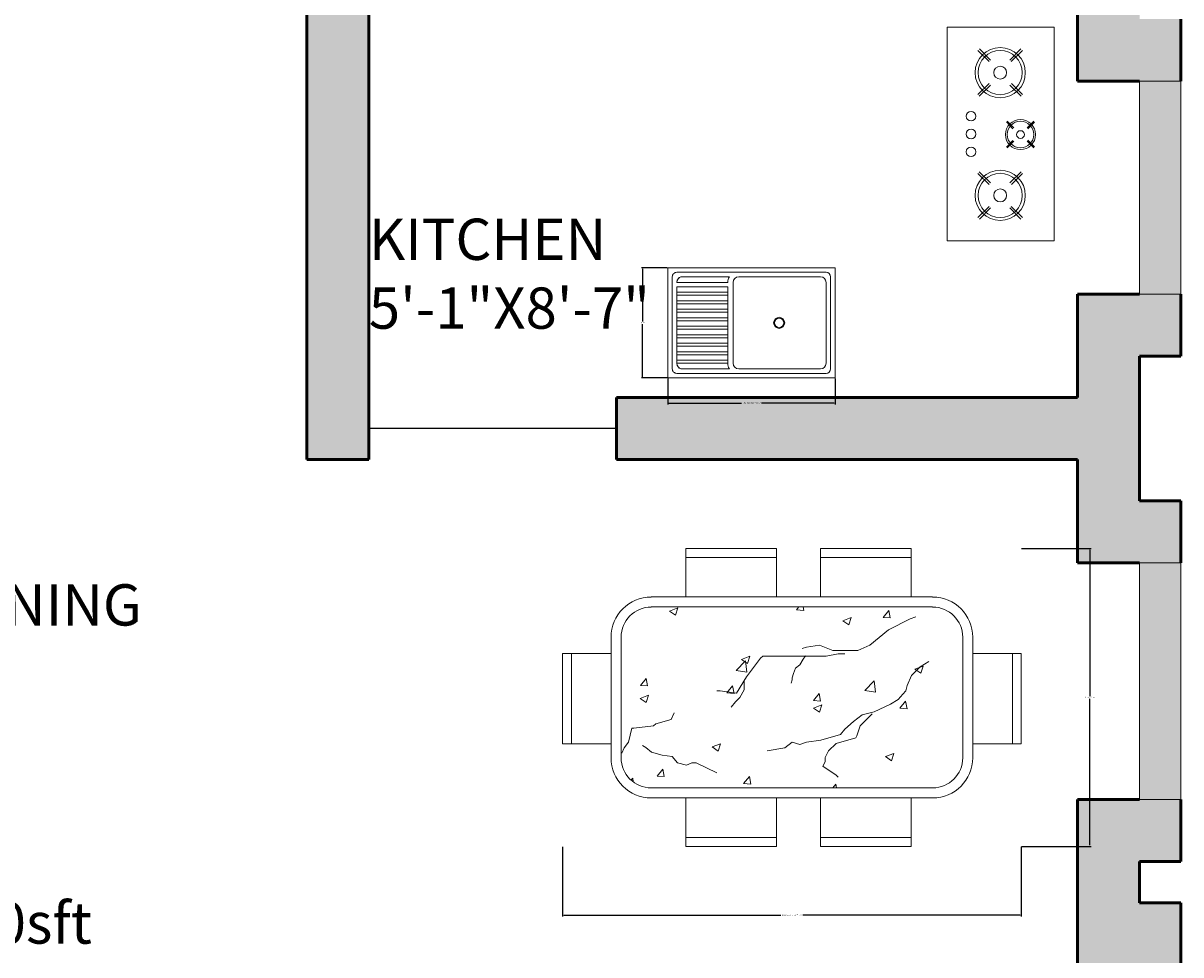
# Model space of a CAD drawing. Units: inches. Extents: x -12 to 604, y -566 to 58.
# Tile 10 of 12: x 436 to 604, y -332 to -196. Entities that reach past the tile are written whole.
import ezdxf

# ---------------------------------------------------------------- set-up
doc = ezdxf.new("R2010")
doc.units = ezdxf.units.IN
doc.header["$MEASUREMENT"] = 0
for name, color, linetype, lineweight in [('A-ANNO-DIMS', 2, 'Continuous', 18), ('A-AREA-IDEN', 7, 'Continuous', 18), ('A-DOOR', 4, 'Continuous', 25), ('A-EQPM', 8, 'Continuous', 18), ('A-FLOR-FIXT', 9, 'Continuous', 18), ('A-FURN', 8, 'Continuous', 18), ('A-GLAZ', 82, 'Continuous', 18), ('A-GLAZ-PATT', 82, 'Continuous', 13), ('A-WALL', 7, 'Continuous', 50), ('A-WALL-PATT', 18, 'Continuous', 13)]:
    doc.layers.add(name, color=color, linetype=linetype, lineweight=lineweight)
doc.styles.get("Standard").update_dxf_attribs({"font": 'arial.ttf'})
doc.dimstyles.get("Standard").update_dxf_attribs({"dimtxt": 0.18, "dimasz": 0.18, "dimexe": 0.18, "dimexo": 0.0625, "dimgap": 0.09, "dimtad": 0, "dimtih": 1, "dimtoh": 1, "dimdec": 0, "dimzin": 0, "dimdsep": 46, "dimlunit": 3, "dimtxsty": 'Standard', "dimcen": 0.09, "dimadec": 0, "dimazin": 0, "dimtfac": 1, "dimtdec": 0, "dimtofl": 0, "dimtmove": 0, "dimatfit": 3, "dimfxl": 1, "dimtolj": 1, "dimtzin": 0, "dimarcsym": 0})

# ---------------------------------------------------------------- blocks, each defined once
blk = doc.blocks.new('М12 540х820')
for p, q in [((0, 540), (-820, 540)), ((-820, 540), (-820, 0)), ((-45, 517.5), (-775, 517.5)), ((0, 0), (0, 540)), ((-797.5, 495), (-797.5, 45)), ((-775, 468), (-775, 72)), ((-347.5, 495), (-748, 495)), ((-320.5, 468), (-320.5, 72)), ((-301.7, 495), (-64.8, 495)), ((-293.7, 468), (-293.7, 472.5)), ((-293.7, 468), (-45, 468)), ((-45, 469.5), (-45, 468)), ((-22.5, 45), (-22.5, 495)), ((-293.7, 446.6), (-45, 446.6)), ((-293.7, 419.6), (-293.7, 446.6)), ((-293.7, 419.6), (-45, 419.6)), ((-293.7, 405), (-45, 405)), ((-293.7, 378), (-293.7, 405)), ((-45, 419.6), (-45, 446.6)), ((-45, 378), (-45, 405)), ((-293.7, 378), (-45, 378)), ((-293.7, 336.4), (-293.7, 363.4)), ((-293.7, 363.4), (-45, 363.4)), ((-45, 336.4), (-45, 363.4)), ((-293.7, 336.4), (-45, 336.4)), ((-293.7, 294.7), (-293.7, 321.7)), ((-293.7, 321.7), (-45, 321.7)), ((-293.7, 294.7), (-45, 294.7)), ((-45, 294.7), (-45, 321.7)), ((-293.7, 253.1), (-293.7, 280.1)), ((-293.7, 280.1), (-45, 280.1)), ((-293.7, 253.1), (-45, 253.1)), ((-293.7, 211.5), (-293.7, 238.5)), ((-293.7, 238.5), (-45, 238.5)), ((-45, 253.1), (-45, 280.1)), ((-45, 211.5), (-45, 238.5)), ((-293.7, 211.5), (-45, 211.5)), ((-293.7, 169.9), (-293.7, 196.9)), ((-293.7, 196.9), (-45, 196.9)), ((-45, 169.9), (-45, 196.9)), ((-293.7, 169.9), (-45, 169.9)), ((-293.7, 128.2), (-293.7, 155.2)), ((-293.7, 155.2), (-45, 155.2)), ((-293.7, 128.2), (-45, 128.2)), ((-293.7, 113.6), (-45, 113.6)), ((-293.7, 86.6), (-293.7, 113.6)), ((-45, 128.2), (-45, 155.2)), ((-45, 86.6), (-45, 113.6)), ((-293.7, 86.6), (-45, 86.6)), ((-293.7, 72), (-45, 72)), ((-45, 70.5), (-45, 72)), ((-820, 0), (0, 0)), ((-775, 22.5), (-45, 22.5)), ((-748, 45), (-347.5, 45)), ((-301.7, 45), (-64.8, 45))]:
    blk.add_line(p, q)
at = {"ltscale": 0.06}
for p, q in [((-820, 0), (-820, 540)), ((-820, 540), (0, 540)), ((0, 540), (0, 536.9)), ((0, 536.9), (0, 0)), ((-293.7, 446.6), (-45, 446.6)), ((-293.7, 405), (-293.7, 446.6)), ((-293.7, 363.4), (-293.7, 405)), ((-45, 446.6), (-45, 419.6)), ((-45, 419.6), (-45, 378)), ((-293.7, 321.7), (-293.7, 363.4)), ((-45, 378), (-45, 336.4)), ((-293.7, 280.1), (-293.7, 321.7)), ((-45, 336.4), (-45, 294.7)), ((-45, 294.7), (-45, 253.1)), ((-293.7, 238.5), (-293.7, 280.1)), ((-293.7, 196.9), (-293.7, 238.5)), ((-45, 253.1), (-45, 211.5)), ((-293.7, 155.2), (-293.7, 196.9)), ((-45, 211.5), (-45, 169.9)), ((-293.7, 113.6), (-293.7, 155.2)), ((-293.7, 72), (-293.7, 113.6)), ((-45, 169.9), (-45, 128.2)), ((-45, 128.2), (-45, 86.6)), ((-45, 72), (-293.7, 72)), ((-45, 86.6), (-45, 72)), ((0, 0), (-820, 0))]:
    blk.add_line(p, q, dxfattribs=at)
at = {"extrusion": (0, 0, -1)}
for centre, major_axis, start_param, end_param in [((-775, 495), (-15.9, 15.9), -0.785398, 0.785398), ((-775, 495), (-15.9, 15.9), -0.785398, 0.785398), ((-45, 495), (-15.9, -15.9), 2.356194, 3.926991), ((-45, 495), (-15.9, -15.9), 2.356194, 3.926991), ((-748, 468), (-19.1, -19.1), 0.785398, 2.356194), ((-748, 468), (-19.1, -19.1), 0.785398, 2.356194), ((-347.5, 468), (-19.1, 19.1), 0.785398, 2.356194), ((-347.5, 468), (-19.1, 19.1), 0.785398, 2.356194), ((-343.2, 468), (-35, 35), 1.779263, 2.356194), ((-343.2, 468), (-35, 35), 1.779263, 2.356192), ((-343.2, 468), (-35, 35), 2.356192, 2.356194), ((-72.3, 468.8), (-19.3, 19.3), 1.0328, 2.38382), ((-72.3, 468.8), (-19.3, 19.3), 1.0328, 1.064673), ((-72.3, 468.8), (-19.3, 19.3), 1.064673, 2.328569), ((-72.3, 468.8), (-19.3, 19.3), 2.328569, 2.38382), ((-545.5, 270), (-19.1, -19.1), 3.926991, 10.210176), ((-545.5, 270), (-19.1, -19.1), 3.926991, 10.210176), ((-545.5, 270), (-15.9, -15.9), 3.926991, 10.210176), ((-545.5, 270), (-15.9, -15.9), 3.926991, 10.210176), ((-748, 72), (-19.1, 19.1), 3.926991, 5.497787), ((-748, 72), (-19.1, 19.1), 3.926991, 5.497787), ((-347.5, 72), (-19.1, -19.1), 3.926991, 5.497787), ((-347.5, 72), (-19.1, -19.1), 3.926991, 5.497787), ((-343.2, 72), (-35, -35), 3.926991, 4.503922), ((-343.2, 72), (-35, -35), 3.926991, 4.503922), ((-72.3, 71.2), (-19.3, -19.3), 3.899365, 5.250385), ((-72.3, 71.2), (-19.3, -19.3), 3.954617, 5.218512), ((-72.3, 71.2), (-19.3, -19.3), 3.899365, 3.954617), ((-775, 45), (-15.9, -15.9), 5.497787, 7.068583), ((-775, 45), (-15.9, -15.9), 5.497787, 7.068583), ((-72.3, 71.2), (-19.3, -19.3), 5.218512, 5.250385), ((-45, 45), (-15.9, 15.9), 2.356194, 3.926991), ((-45, 45), (-15.9, 15.9), 2.356194, 3.926991)]:
    blk.add_ellipse(centre, major_axis=major_axis, ratio=1, start_param=start_param, end_param=end_param, dxfattribs=at)
blk = doc.blocks.new('DINING-TABLE-6-SEAT')
for p, q in [((17.93, 36.25), (17.93, 43.28)), ((17.93, 43.28), (31.08, 43.28)), ((31.08, 43.28), (31.08, 36.25)), ((37.5, 36.25), (37.5, 43.28)), ((37.5, 43.28), (50.64, 43.28)), ((50.64, 43.28), (50.64, 36.25)), ((31.08, 42), (17.93, 42)), ((50.64, 42), (37.5, 42)), ((53.77, 36.25), (12.88, 36.25)), ((12.88, 34.79), (53.77, 34.79)), ((15.53, 34.2), (16.76, 34.67)), ((15.53, 34.2), (16.41, 33.61)), ((16.41, 33.61), (16.76, 34.67)), ((34.01, 34.38), (34.34, 34.79)), ((34.01, 34.38), (35.05, 34.29)), ((35.05, 34.29), (34.96, 34.79)), ((46.57, 33.28), (47.42, 34.29)), ((47.62, 33.19), (47.42, 34.29)), ((40.72, 32.8), (41.94, 33.27)), ((40.72, 32.8), (41.59, 32.21)), ((41.59, 32.21), (41.95, 33.27)), ((46.57, 33.28), (47.62, 33.19)), ((50.53, 33.06), (47.35, 31.47)), ((51.32, 33.37), (50.53, 33.06)), ((7.04, 30.4), (7.04, 12.88)), ((8.5, 12.88), (8.5, 30.4)), ((47.35, 31.47), (44.66, 29.25)), ((58.15, 30.4), (58.15, 12.88)), ((59.61, 12.88), (59.61, 30.4)), ((35.45, 28.93), (34.81, 28.77)), ((37.35, 29.25), (35.45, 28.93)), ((39.26, 28.46), (37.35, 29.25)), ((44.66, 29.25), (42.91, 28.46)), ((0, 28.04), (0, 14.9)), ((7.04, 28.04), (0, 28.04)), ((1.29, 14.9), (1.29, 28.04)), ((25.21, 25.55), (26.57, 26.98)), ((25.99, 27.15), (27.22, 27.62)), ((25.99, 27.15), (26.87, 26.56)), ((26.76, 25.31), (26.57, 26.98)), ((28.78, 27.35), (26.71, 24.65)), ((26.87, 26.56), (27.22, 27.62)), ((29.09, 27.66), (28.78, 27.35)), ((38.3, 27.66), (29.09, 27.66)), ((34.97, 27.19), (34.49, 26.4)), ((35.29, 27.67), (34.97, 27.19)), ((40.05, 27.98), (38.3, 27.66)), ((42.91, 28.46), (39.26, 28.46)), ((41, 27.98), (40.05, 27.98)), ((66.65, 28.04), (59.61, 28.04)), ((65.37, 28.04), (65.37, 14.9)), ((66.65, 14.9), (66.65, 28.04)), ((25.21, 25.55), (26.76, 25.31)), ((33.86, 25.92), (33.54, 25.13)), ((34.49, 26.4), (33.86, 25.92)), ((51.96, 26.08), (50.69, 24.81)), ((51.18, 25.74), (52.41, 26.21)), ((51.18, 25.74), (52.05, 25.15)), ((53.23, 26.87), (51.96, 26.08)), ((52.05, 25.15), (52.41, 26.21)), ((11.3, 23.4), (12.14, 24.41)), ((12.35, 23.31), (12.14, 24.41)), ((26.71, 24.65), (25.28, 22.27)), ((26.39, 24.17), (26.39, 22.75)), ((33.38, 24.18), (33.22, 23.7)), ((33.54, 25.13), (33.38, 24.5)), ((33.38, 24.5), (33.38, 24.18)), ((43.91, 22.65), (45.27, 24.08)), ((45.47, 22.41), (45.27, 24.07)), ((50.69, 24.81), (50.05, 23.38)), ((11.27, 21.49), (12.5, 21.97)), ((11.3, 23.4), (12.35, 23.31)), ((12.14, 20.91), (12.5, 21.96)), ((22.9, 22.59), (22.42, 22.59)), ((25.28, 22.27), (22.9, 22.59)), ((23.87, 22.3), (24.71, 23.31)), ((23.87, 22.3), (24.91, 22.21)), ((24.92, 22.21), (24.71, 23.31)), ((26.39, 22.75), (25.76, 21.64)), ((36.44, 21.2), (37.28, 22.21)), ((37.48, 21.11), (37.28, 22.21)), ((43.91, 22.65), (45.47, 22.41)), ((49.42, 22.11), (48.78, 21.32)), ((49.9, 22.59), (49.42, 22.11)), ((50.05, 23.38), (49.9, 22.59)), ((11.27, 21.49), (12.14, 20.91)), ((25.12, 21), (24.49, 20.21)), ((25.76, 21.64), (25.12, 21)), ((36.44, 21.2), (37.48, 21.11)), ((36.45, 20.09), (37.68, 20.56)), ((37.33, 19.5), (37.68, 20.56)), ((47.67, 20.68), (45.29, 19.57)), ((48.78, 21.32), (47.67, 20.68)), ((49.01, 20.1), (49.85, 21.11)), ((50.05, 20.01), (49.85, 21.11)), ((15.76, 18.46), (16.23, 19.41)), ((36.45, 20.09), (37.33, 19.5)), ((43.54, 19.1), (42.27, 18.15)), ((44.34, 18.62), (43.23, 17.51)), ((45.29, 19.57), (43.54, 19.1)), ((44.97, 19.26), (44.34, 18.62)), ((49.01, 20.1), (50.05, 20.01)), ((9.56, 15.13), (10.04, 17.19)), ((10.04, 17.19), (10.36, 17.19)), ((10.36, 17.19), (13.21, 17.51)), ((13.21, 17.51), (13.53, 17.83)), ((13.53, 17.83), (15.76, 18.46)), ((41, 17.04), (40.37, 16.24)), ((42.27, 18.15), (41, 17.04)), ((43.23, 17.51), (42.75, 16.08)), ((37.51, 15.45), (35.45, 15.13)), ((40.37, 16.24), (37.51, 15.45)), ((42.59, 15.77), (39.73, 14.97)), ((42.75, 16.08), (42.59, 15.77)), ((0, 14.9), (7.04, 14.9)), ((8.61, 13.55), (8.93, 14.34)), ((8.93, 14.34), (9.56, 15.13)), ((12.11, 14.35), (11.63, 14.66)), ((12.9, 13.71), (12.11, 14.35)), ((14.49, 13.23), (12.9, 13.71)), ((21.73, 14.44), (22.96, 14.91)), ((21.73, 14.44), (22.6, 13.85)), ((22.6, 13.85), (22.96, 14.91)), ((32.27, 14.34), (29.73, 13.86)), ((33.38, 15.13), (32.27, 14.34)), ((34.49, 14.82), (33.38, 15.13)), ((35.45, 15.13), (34.49, 14.82)), ((38.62, 13.86), (38.14, 12.91)), ((39.73, 14.97), (38.62, 13.86)), ((46.91, 13.04), (48.14, 13.51)), ((47.79, 12.45), (48.14, 13.51)), ((59.61, 14.9), (66.65, 14.9)), ((15.92, 13.08), (14.49, 13.23)), ((16.71, 12.12), (15.92, 13.08)), ((17.98, 11.81), (16.71, 12.12)), ((18.77, 12.12), (17.98, 11.81)), ((19.41, 12.12), (18.77, 12.12)), ((22.43, 10.7), (19.41, 12.12)), ((38.14, 12.28), (37.83, 11.64)), ((38.14, 12.91), (38.14, 12.28)), ((46.91, 13.04), (47.79, 12.45)), ((13.73, 10.22), (14.57, 11.23)), ((13.73, 10.22), (14.78, 10.13)), ((14.78, 10.13), (14.57, 11.23)), ((26.3, 9.12), (27.14, 10.13)), ((27.35, 9.03), (27.14, 10.13)), ((37.83, 11.64), (39.73, 10.37)), ((39.73, 10.37), (40.05, 10.06)), ((9.93, 9.64), (10.19, 9.91)), ((10.25, 9.37), (10.19, 9.9)), ((53.77, 8.5), (12.88, 8.5)), ((26.3, 9.12), (27.35, 9.03)), ((39.27, 8.5), (39.71, 9.03)), ((39.81, 8.5), (39.71, 9.03)), ((12.88, 7.04), (53.77, 7.04)), ((17.93, 7.04), (17.93, 0)), ((31.08, 0), (31.08, 7.04)), ((37.5, 7.04), (37.5, 0)), ((50.64, 0), (50.64, 7.04)), ((31.08, 1.29), (17.93, 1.29)), ((50.64, 1.29), (37.5, 1.29)), ((17.93, 0), (31.08, 0)), ((37.5, 0), (50.64, 0))]:
    blk.add_line(p, q)
for centre, radius, start, end in [((12.88, 30.4), 5.84, 90, 180), ((53.77, 30.4), 5.84, 0, 90), ((12.88, 30.4), 4.38, 90, 180), ((53.77, 30.4), 4.38, 0, 90), ((12.88, 12.88), 5.84, 180, 270), ((12.88, 12.88), 4.38, 180, 270), ((53.77, 12.88), 4.38, 270, 0), ((53.77, 12.88), 5.84, 270, 0)]:
    blk.add_arc(centre, radius, start, end)
blk = doc.blocks.new('*D19')
at = {"layer": 'A-ANNO-DIMS', "color": 0, "lineweight": -2, "transparency": 16777216}
for p, q in [((529.75, -248.08), (529.75, -251.85)), ((554.1, -248.08), (554.1, -251.85)), ((529.93, -251.67), (540.48, -251.67)), ((553.92, -251.67), (543.38, -251.67))]:
    blk.add_line(p, q, dxfattribs=at)
at = {"layer": 'A-ANNO-DIMS', "color": 0, "transparency": 16777216}
for points in [[(529.93, -251.64), (529.93, -251.7), (529.75, -251.67)], [(553.92, -251.64), (553.92, -251.7), (554.1, -251.67)]]:
    blk.add_solid(points, dxfattribs=at)
at = {"layer": 'Defpoints', "color": 0, "transparency": 16777216}
for p in [(529.75, -248.02), (554.1, -248.02), (529.75, -251.67)]:
    blk.add_point(p, dxfattribs=at)
at = {"layer": 'A-ANNO-DIMS', "color": 0, "transparency": 16777216, "insert": (541.93, -251.67), "char_height": 0.18, "attachment_point": 5}
blk.add_mtext('\\A1;KITCHEN SINK 2\'-0 1/2"', dxfattribs=at)
blk = doc.blocks.new('*D20')
at = {"layer": 'A-ANNO-DIMS', "color": 0, "lineweight": -2, "transparency": 16777216}
for p, q in [((529.69, -231.99), (525.92, -231.99)), ((526.1, -232.17), (526.1, -239.82)), ((526.1, -247.84), (526.1, -240.18)), ((529.69, -248.02), (525.92, -248.02))]:
    blk.add_line(p, q, dxfattribs=at)
at = {"layer": 'A-ANNO-DIMS', "color": 0, "transparency": 16777216}
for points in [[(526.07, -232.17), (526.13, -232.17), (526.1, -231.99)], [(526.07, -247.84), (526.13, -247.84), (526.1, -248.02)]]:
    blk.add_solid(points, dxfattribs=at)
at = {"layer": 'Defpoints', "color": 0, "transparency": 16777216}
for p in [(526.1, -231.99), (529.75, -231.99), (529.75, -248.02)]:
    blk.add_point(p, dxfattribs=at)
at = {"layer": 'A-ANNO-DIMS', "color": 0, "transparency": 16777216, "insert": (526.1, -240), "char_height": 0.18, "attachment_point": 5}
blk.add_mtext('\\A1;1\'-4"', dxfattribs=at)
blk = doc.blocks.new('*D29')
at = {"layer": 'A-ANNO-DIMS', "color": 0, "lineweight": -2, "transparency": 16777216}
for p, q in [((514.48, -316.15), (514.48, -326.27)), ((581.13, -316.15), (581.13, -326.27)), ((514.66, -326.09), (546.2, -326.09)), ((580.95, -326.09), (549.4, -326.09))]:
    blk.add_line(p, q, dxfattribs=at)
at = {"layer": 'A-ANNO-DIMS', "color": 0, "transparency": 16777216}
for points in [[(514.66, -326.06), (514.66, -326.12), (514.48, -326.09)], [(580.95, -326.06), (580.95, -326.12), (581.13, -326.09)]]:
    blk.add_solid(points, dxfattribs=at)
at = {"layer": 'Defpoints', "color": 0, "transparency": 16777216}
for p in [(514.48, -316.09), (581.13, -316.09), (581.13, -326.09)]:
    blk.add_point(p, dxfattribs=at)
at = {"layer": 'A-ANNO-DIMS', "color": 0, "transparency": 16777216, "insert": (547.8, -326.09), "char_height": 0.18, "attachment_point": 5}
blk.add_mtext('\\A1;DINING SET 5\'-6 1/2" TYP.', dxfattribs=at)
blk = doc.blocks.new('*D30')
at = {"layer": 'A-ANNO-DIMS', "color": 0, "lineweight": -2, "transparency": 16777216}
for p, q in [((581.19, -272.8), (591.3, -272.8)), ((591.12, -272.98), (591.12, -294.26)), ((591.12, -315.91), (591.12, -294.63)), ((581.19, -316.09), (591.3, -316.09))]:
    blk.add_line(p, q, dxfattribs=at)
at = {"layer": 'A-ANNO-DIMS', "color": 0, "transparency": 16777216}
for points in [[(591.09, -272.98), (591.15, -272.98), (591.12, -272.8)], [(591.09, -315.91), (591.15, -315.91), (591.12, -316.09)]]:
    blk.add_solid(points, dxfattribs=at)
at = {"layer": 'Defpoints', "color": 0, "transparency": 16777216}
for p in [(581.13, -272.8), (591.12, -272.8), (581.13, -316.09)]:
    blk.add_point(p, dxfattribs=at)
at = {"layer": 'A-ANNO-DIMS', "color": 0, "transparency": 16777216, "insert": (591.12, -294.45), "char_height": 0.18, "attachment_point": 5}
blk.add_mtext('\\A1;3\'-7 1/2" TYP.', dxfattribs=at)

msp = doc.modelspace()

# ---------------------------------------------------------------- hatches: boundary and pattern name
at = {"layer": 'A-GLAZ-PATT'}
h = msp.add_hatch(dxfattribs=at)
h.set_pattern_fill('GOST_WOOD', color=256)
h.set_pattern_definition([(90, (0, 0), (6, -4e-16), [10, -2]), (90, (2, -2), (6, -4e-16), [6, -1.5, 3, -1.5]), (90, (4, -5), (6, -4e-16), [10, -2])])
h.paths.add_polyline_path([(344.32, -529.86), (344.32, -520.86), (284.32, -520.86), (284.32, -529.86)])
h.paths.add_polyline_path([(604.32, -450.86), (598.32, -450.86), (598.32, -474.86), (604.32, -474.86)])
h.paths.add_polyline_path([(598.32, -309.28), (604.32, -309.28), (604.32, -274.86), (598.32, -274.86)])
h.paths.add_polyline_path([(598.32, -235.86), (604.32, -235.86), (604.32, -204.86), (598.32, -204.86)])
h.paths.add_polyline_path([(598.32, -159.86), (604.32, -159.86), (604.32, -99.86), (598.32, -99.86)])
at = {"layer": 'A-WALL-PATT'}
h = msp.add_hatch(color=256, dxfattribs=at)
h.dxf.hatch_style = 1
h.paths.add_polyline_path([(169.32, 11.14), (169.32, 17.14), (160.32, 17.14), (160.32, 11.14), (118.32, 11.14), (118.32, 6.64), (118.32, 2.14), (127.32, 2.14), (169.32, 2.14)])
h.paths.add_polyline_path([(127.32, -13.61), (118.32, -13.61), (118.32, -29.36), (34.82, -29.36), (24.32, -29.36), (24.32, -38.36), (39.32, -38.36), (118.32, -38.36), (118.32, -126.86), (127.32, -126.86), (127.32, -117.86)])
h.paths.add_polyline_path([(82.32, -92.36), (39.32, -92.36), (39.32, -56.22), (30.32, -56.22), (24.32, -56.22), (24.32, -65.22), (30.32, -65.22), (30.32, -113.36), (24.32, -113.36), (24.32, -122.36), (39.32, -122.36), (39.32, -101.36), (82.32, -101.36), (82.32, -96.86)], flags=17)
h.paths.add_polyline_path([(280.32, 11.14), (238.32, 11.14), (238.32, 17.14), (229.32, 17.14), (229.32, 12.64), (229.32, 11.14), (229.32, 2.14), (271.32, 2.14), (271.32, -117.86), (163.32, -117.86), (163.32, -126.86), (271.32, -126.86), (271.32, -189.86), (280.32, -189.86), (280.32, -180.86)])
h.paths.add_polyline_path([(415.32, 17.14), (406.32, 17.14), (406.32, 11.14), (358.32, 11.14), (358.32, -21.86), (367.32, -21.86), (367.32, 2.14), (415.32, 2.14)], flags=17)
h.paths.add_polyline_path([(484.55, -45.86), (448.32, -45.86), (448.32, 2.14), (448.32, 17.14), (439.32, 17.14), (439.32, 12.64), (439.32, 2.14), (439.32, -45.86), (367.32, -45.86), (358.32, -45.86), (358.32, -54.86), (430.32, -54.86), (430.32, -69.59), (430.32, -180.86), (318.82, -180.86), (318.82, -189.86), (318.82, -331.86), (327.82, -331.86), (327.82, -189.86), (439.32, -189.86), (439.32, -180.86), (439.32, -54.86), (483.5, -54.86), (484.55, -54.86)])
h.paths.add_polyline_path([(529.32, 11.14), (481.32, 11.14), (481.32, 17.14), (472.32, 17.14), (472.32, 12.64), (472.32, 2.14), (520.32, 2.14), (520.32, -21.86), (529.32, -21.86)])
h.paths.add_polyline_path([(598.32, -45.86), (582.42, -45.86), (582.42, -50.36), (582.42, -54.86), (589.32, -54.86), (589.32, -99.86), (598.32, -99.86), (604.32, -99.86), (604.32, -90.86), (598.32, -90.86)])
h.paths.add_polyline_path([(598.32, -168.86), (604.32, -168.86), (604.32, -159.86), (589.32, -159.86), (589.32, -180.86), (477.32, -180.86), (477.32, -189.86), (477.32, -259.86), (486.32, -259.86), (486.32, -189.86), (589.32, -189.86), (589.32, -204.86), (598.32, -204.86), (604.32, -204.86), (604.32, -195.86), (598.32, -195.86)])
h.paths.add_polyline_path([(598.32, -244.86), (604.32, -244.86), (604.32, -235.86), (598.32, -235.86), (589.32, -235.86), (589.32, -250.86), (522.32, -250.86), (522.32, -259.86), (589.32, -259.86), (589.32, -274.86), (598.32, -274.86), (604.32, -274.86), (604.32, -265.86), (598.32, -265.86)])
h.paths.add_polyline_path([(598.32, -333.28), (604.32, -333.28), (604.32, -324.28), (598.32, -324.28), (598.32, -321.87), (598.32, -318.28), (604.32, -318.28), (604.32, -309.28), (598.32, -309.28), (589.32, -309.28), (589.32, -341.95), (589.38, -341.95), (589.38, -363.16), (589.32, -381.86), (565.32, -381.86), (565.32, -390.86), (589.32, -390.86), (589.32, -450.86), (598.32, -450.86), (604.32, -450.86), (604.32, -441.86), (598.32, -441.86), (598.32, -390.86), (604.32, -390.86), (604.32, -381.86), (598.32, -381.86)])
h.paths.add_polyline_path([(541.32, -345.86), (424.32, -345.86), (424.32, -354.86), (532.32, -354.86), (532.32, -474.86), (463.39, -474.86), (463.39, -483.86), (553.32, -483.86), (553.32, -474.86), (541.32, -474.86), (541.32, -390.86), (541.32, -381.86)])
h.paths.add_polyline_path([(604.32, -474.86), (589.32, -474.86), (553.32, -474.86), (553.32, -483.86), (598.32, -483.86), (604.32, -483.86)])
h.paths.add_polyline_path([(388.32, -483.86), (388.32, -474.86), (388.32, -460.13), (388.32, -333.86), (388.32, -322.86), (379.32, -322.86), (379.32, -331.86), (379.32, -333.86), (379.32, -474.86), (379.32, -520.86), (344.32, -520.86), (344.32, -529.86), (379.32, -529.86), (388.32, -529.86)])
h.paths.add_polyline_path([(284.32, -520.86), (249.32, -520.86), (249.32, -474.86), (249.32, -368.36), (240.32, -368.36), (240.32, -474.86), (238.52, -474.86), (238.52, -483.86), (240.32, -483.86), (240.32, -529.86), (249.32, -529.86), (284.32, -529.86)])
h.paths.add_polyline_path([(178.82, -474.86), (158.91, -474.86), (158.91, -483.86), (162.32, -483.86), (178.82, -483.86)])
h.paths.add_polyline_path([(84.32, -474.86), (84.32, -366.86), (75.32, -366.86), (75.32, -474.86), (39.32, -474.86), (39.32, -453.86), (24.32, -453.86), (24.32, -462.86), (30.32, -462.86), (30.32, -483.86), (84.32, -483.86)])
h.paths.add_polyline_path([(39.32, -342.86), (75.32, -342.86), (84.32, -342.86), (179.67, -342.86), (179.67, -333.86), (39.32, -333.86), (39.32, -318.86), (24.32, -318.86), (24.32, -327.86), (30.32, -327.86), (30.32, -432.86), (24.32, -432.86), (24.32, -441.86), (30.32, -441.86), (39.32, -441.86)])
h.paths.add_polyline_path([(249.32, -252.86), (115.32, -252.86), (115.32, -225.86), (106.32, -225.86), (106.32, -252.86), (39.32, -252.86), (39.32, -237.86), (24.32, -237.86), (24.32, -246.86), (30.32, -246.86), (30.32, -267.86), (24.32, -267.86), (24.32, -276.86), (39.32, -276.86), (39.32, -261.86), (240.32, -261.86), (240.32, -331.86), (249.32, -331.86), (266.82, -331.86), (266.82, -322.86), (249.32, -322.86)])
h.paths.add_polyline_path([(127.32, -180.86), (39.32, -180.86), (24.32, -180.86), (24.32, -189.86), (39.32, -189.86), (127.32, -189.86)])
h.paths.add_polyline_path([(39.32, -159.86), (24.32, -159.86), (24.32, -168.86), (30.32, -168.86), (30.32, -180.86), (39.32, -180.86)])
h.paths.add_polyline_path([(470.51, -17.27), (512.48, -17.27), (512.48, 5.12), (470.51, 5.12)], flags=9)
h.paths.add_polyline_path([(484.21, -244.26), (526.45, -244.26), (526.45, -221.87), (484.21, -221.87)], flags=24)
h.paths.add_polyline_path([(36.91, -442.88), (83.54, -442.88), (83.54, -420.5), (36.91, -420.5)], flags=25)

# ---------------------------------------------------------------- linework, layer by layer
at = {"layer": 'A-DOOR'}
msp.add_line((522.32, -255.36), (486.32, -255.36), dxfattribs=at)
at = {"layer": 'A-EQPM'}
for p, q in [((570.38, -228.08), (570.38, -197.04)), ((570.38, -197.04), (585.9, -197.04)), ((585.9, -197.04), (585.9, -228.08)), ((576.67, -201.82), (575.06, -200.2)), ((579.46, -201.82), (581.08, -200.2)), ((576.46, -202.03), (574.84, -200.42)), ((579.68, -202.03), (581.29, -200.42)), ((576.45, -205.24), (574.82, -206.84)), ((579.69, -205.24), (581.32, -206.84)), ((576.66, -205.46), (575.03, -207.06)), ((579.48, -205.46), (581.11, -207.06)), ((579.93, -211.79), (578.97, -210.81)), ((580.06, -211.66), (579.1, -210.68)), ((581.98, -211.67), (582.95, -210.7)), ((582.11, -211.8), (583.08, -210.83)), ((579.93, -213.48), (578.97, -214.46)), ((580.06, -213.61), (579.1, -214.59)), ((581.98, -213.6), (582.95, -214.57)), ((582.11, -213.47), (583.08, -214.44)), ((576.45, -219.88), (574.82, -218.28)), ((576.66, -219.66), (575.03, -218.06)), ((579.48, -219.66), (581.11, -218.06)), ((579.69, -219.88), (581.32, -218.28)), ((576.46, -223.09), (574.84, -224.7)), ((576.67, -223.3), (575.06, -224.92)), ((579.46, -223.3), (581.08, -224.92)), ((579.68, -223.09), (581.29, -224.7)), ((585.9, -228.08), (570.38, -228.08))]:
    msp.add_line(p, q, dxfattribs=at)
for centre, radius in [((578.07, -203.64), 3.65), ((578.07, -203.64), 3.21), ((578.07, -203.64), 0.94), ((573.83, -209.97), 0.69), ((573.83, -212.56), 0.69), ((581.02, -212.64), 2.19), ((581.02, -212.64), 1.93), ((581.02, -212.64), 0.564), ((573.83, -215.15), 0.69), ((578.07, -221.48), 3.65), ((578.07, -221.48), 3.21), ((578.07, -221.48), 0.94)]:
    msp.add_circle(centre, radius, dxfattribs=at)
at = {"layer": 'A-GLAZ'}
for p, q in [((598.32, -204.86), (604.32, -204.86)), ((598.32, -235.86), (598.32, -204.86)), ((604.32, -204.86), (604.32, -235.86)), ((598.32, -235.86), (604.32, -235.86)), ((598.32, -274.86), (604.32, -274.86)), ((598.32, -309.28), (598.32, -274.86)), ((604.32, -274.86), (604.32, -309.28)), ((598.32, -309.28), (604.32, -309.28))]:
    msp.add_line(p, q, dxfattribs=at)
at = {"layer": 'A-WALL'}
for p, q in [((477.32, -189.86), (477.32, -259.86)), ((486.32, -189.86), (486.32, -259.86)), ((589.32, -189.86), (589.32, -204.86)), ((604.32, -204.86), (604.32, -195.86)), ((589.32, -204.86), (598.32, -204.86)), ((589.32, -235.86), (598.32, -235.86)), ((589.32, -235.86), (589.32, -250.86)), ((604.32, -244.86), (604.32, -235.86)), ((598.32, -244.86), (604.32, -244.86)), ((598.32, -244.86), (598.32, -265.86)), ((522.32, -250.86), (589.32, -250.86)), ((522.32, -250.86), (522.32, -259.86)), ((477.32, -259.86), (486.32, -259.86)), ((522.32, -259.86), (589.32, -259.86)), ((589.32, -259.86), (589.32, -274.86)), ((598.32, -265.86), (604.32, -265.86)), ((604.32, -274.86), (604.32, -265.86)), ((589.32, -274.86), (598.32, -274.86)), ((589.32, -309.28), (589.32, -381.86)), ((598.32, -309.28), (589.32, -309.28)), ((604.32, -318.28), (604.32, -309.28)), ((598.32, -318.28), (604.32, -318.28)), ((598.32, -318.28), (598.32, -321.87)), ((598.32, -321.87), (598.32, -324.28)), ((598.32, -324.28), (604.32, -324.28)), ((604.32, -333.28), (604.32, -324.28))]:
    msp.add_line(p, q, dxfattribs=at)

# ---------------------------------------------------------------- block references
at = {"layer": 'A-FLOR-FIXT', "xscale": -0.0296924051348044, "yscale": 0.0296924051348044, "zscale": 0.0296924051348044}
msp.add_blockref('М12 540х820', (529.75, -248.02), dxfattribs=at)
at = {"layer": 'A-FURN'}
msp.add_blockref('DINING-TABLE-6-SEAT', (514.48, -316.09), dxfattribs=at)

# ---------------------------------------------------------------- texts
at = {"layer": 'A-AREA-IDEN', "char_height": 6, "attachment_point": 1}
for s, insert in [('KITCHEN\\P5\'-1"X8\'-7"', (486.32, -224.86)), ('DRAWING/DINING\\P13\'-5"X19\'-0"', (385.25, -278)), ('UNIT 1\\PAREA=750sft', (398.35, -314.23))]:
    msp.add_mtext(s, dxfattribs=dict(at, insert=insert))

# ---------------------------------------------------------------- dimensions: what is measured, and where the dimension line sits
at = {"layer": 'A-ANNO-DIMS'}
dim = msp.add_linear_dim(base=(526.1, -231.99), p1=(529.75, -248.02), p2=(529.75, -231.99), angle=90, dimstyle='Standard', override={"dimdec": 1, "dimlfac": 1, "dimrnd": 0, "dimzin": 1, "dimdsep": 46, "dimlunit": 4, "dimfrac": 2}, dxfattribs=at)
dim.commit()
dim.dimension.update_dxf_attribs({"geometry": '*D20', "text_midpoint": (526.1, -240)})
for base, p1, p2, angle, text, picture, middle in [((529.7514, -251.6721), (554.0992, -248.0199), (529.7514, -248.0199), 180, 'KITCHEN SINK <>', '*D19', (541.9253, -251.6721)), ((591.12, -272.8), (581.13, -316.09), (581.13, -272.8), 90, '<> TYP.', '*D30', (591.12, -294.45))]:
    dim = msp.add_linear_dim(base=base, p1=p1, p2=p2, angle=angle, text=text, dimstyle='Standard', override={"dimdec": 1, "dimlfac": 1, "dimrnd": 0, "dimzin": 1, "dimdsep": 46, "dimlunit": 4, "dimfrac": 2}, dxfattribs=at)
    dim.commit()
    dim.dimension.update_dxf_attribs({"geometry": picture, "text_midpoint": middle})
dim = msp.add_linear_dim(base=(581.127, -326.0869), p1=(514.4766, -316.0894), p2=(581.127, -316.0894), text='DINING SET <> TYP.', dimstyle='Standard', override={"dimdec": 1, "dimlfac": 1, "dimrnd": 0, "dimzin": 1, "dimdsep": 46, "dimlunit": 4, "dimfrac": 2}, dxfattribs=at)
dim.commit()
dim.dimension.update_dxf_attribs({"geometry": '*D29', "text_midpoint": (547.8018, -326.0869)})

doc.saveas('drawing.dxf')
